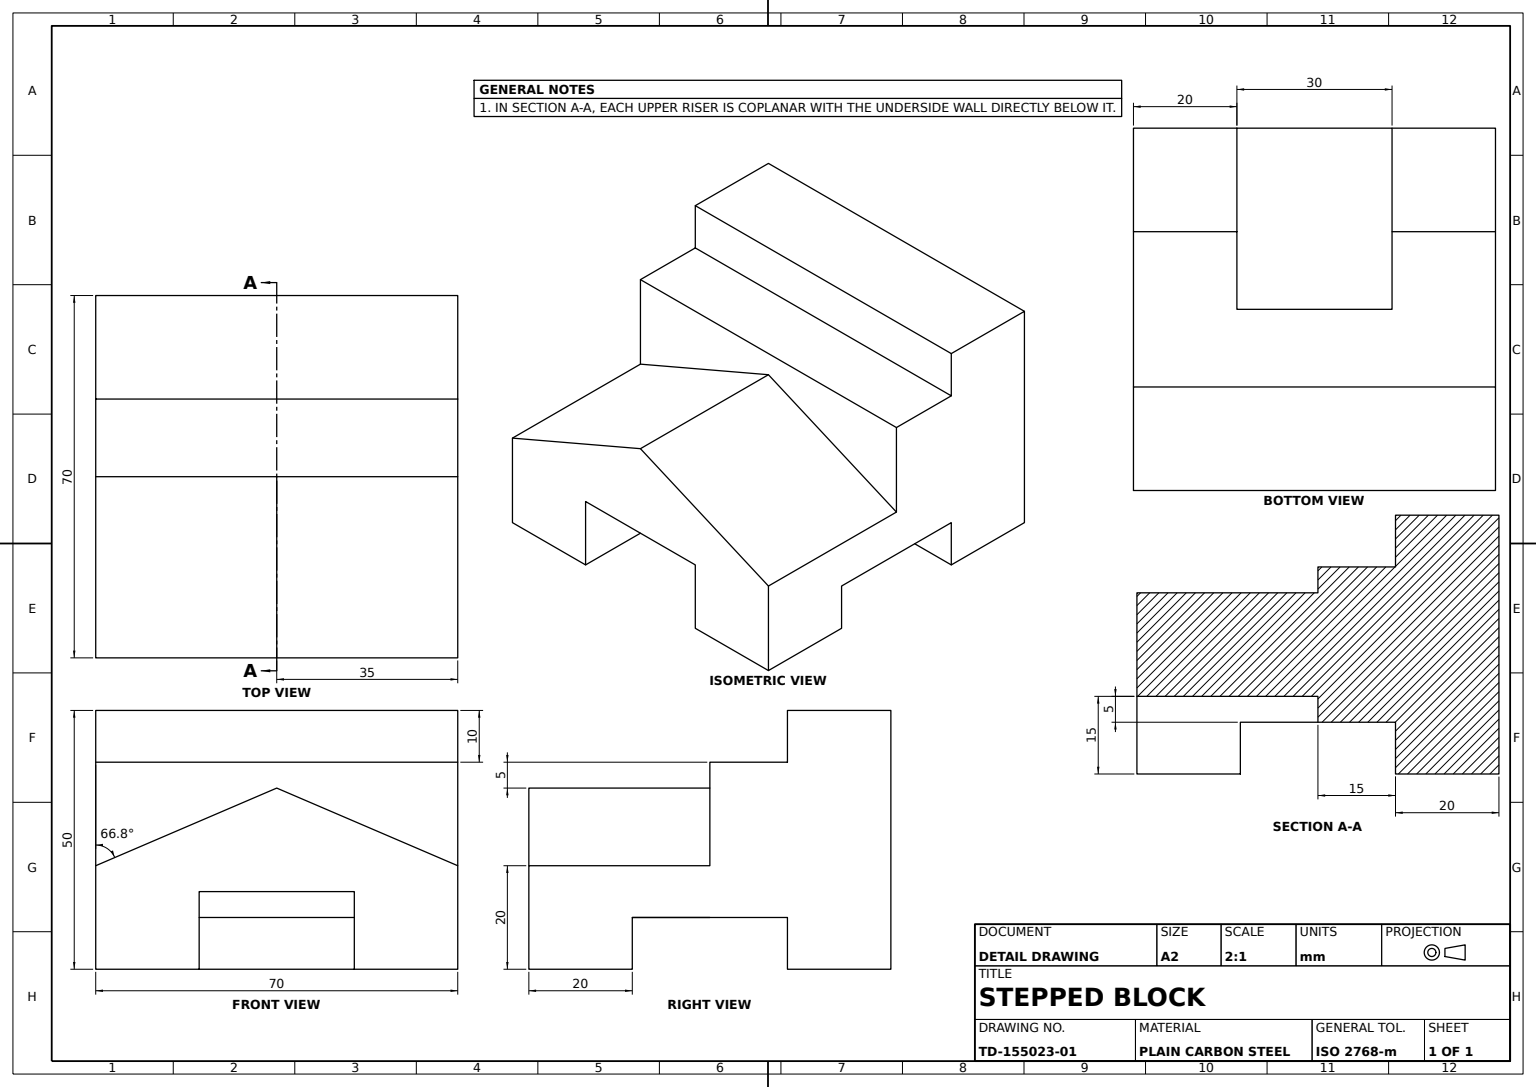
SolidWorks part; units mm, degrees
material "Plain Carbon Steel"
ref_plane "Front Plane" through (0, 0, 0) normal (0, 0, 1) x (1, 0, 0)
ref_plane "Top Plane" through (0, 0, 0) normal (0, 1, 0) x (1, 0, 0)
ref_plane "Right Plane" through (0, 0, 0) normal (1, 0, 0) x (0, 0, -1)
sketch "Base Block Sketch" plane through (0, 0, 0) normal (0, 0, 1) x (1, 0, 0)
  line L0 (0, 0) -> (0, 50)
  line L1 (0, 50) -> (70, 50)
  line L2 (70, 50) -> (70, 0)
  line L3 (70, 0) -> (0, 0)
  dimension "D1" = 70
  dimension "D2" = 50
extrude "Base Block" add sketch "Base Block Sketch" along normal blind 15
sketch "Pad Sketch" plane through (0, 0, 15) normal (0, 0, 1) x (1, 0, 0)
  line L0 (0, 50) -> (70, 50)
  line L1 (70, 50) -> (70, 0)
  line L2 (70, 0) -> (0, 0)
  line L3 (0, 0) -> (0, 50)
extrude "Pad 5mm" add sketch "Pad Sketch" along normal blind 5
sketch "Stepped Profile Sketch" plane through (0, 0, 0) normal (-1, 0, 0) x (0, 0, 1)
  line L0 (0, 50) -> (0, 0) construction
  line L1 (20, 50) -> (20, 0) construction
  line L2 (20, 40) -> (35, 40)
  line L3 (20, 0) -> (0, 0) construction
  line L4 (20, 10) -> (50, 10)
  line L5 (50, 10) -> (50, 0)
  line L6 (50, 0) -> (70, 0)
  line L7 (70, 0) -> (70, 20)
  line L8 (70, 20) -> (35, 20)
  line L9 (35, 20) -> (35, 40)
  line L10 (20, 40) -> (20, 10)
  dimension "D1" = 35
  dimension "D2" = 50
  dimension "D3" = 70
  dimension "D4" = 10
extrude "Stepped Body" add sketch "Stepped Profile Sketch" against normal blind 70
sketch "Wedge Sketch" plane through (0, 0, 70) normal (0, 0, 1) x (1, 0, 0)
  line L1 (70, 0) -> (0, 0) construction
  line L2 (35, 35) -> (0, 20)
  line L3 (0, 20) -> (70, 20)
  line L4 (70, 20) -> (35, 35)
  dimension "D1" = 35
extrude "Angled Wedge" add sketch "Wedge Sketch" against normal blind 35
sketch "Slot Cut Sketch" plane through (0, 0, 70) normal (0, 0, 1) x (1, 0, 0)
  line L0 (35, 0) -> (20, 0)
  line L1 (70, 0) -> (0, 0) construction
  line L2 (20, 0) -> (20, 15)
  line L3 (20, 15) -> (50, 15)
  line L4 (50, 15) -> (50, 0)
  line L5 (50, 0) -> (35, 0)
  line L6 (0, 0) -> (0, 20) construction
  dimension "D1" = 20
extrude "Front Slot Cut" cut sketch "Slot Cut Sketch" against normal blind 35
